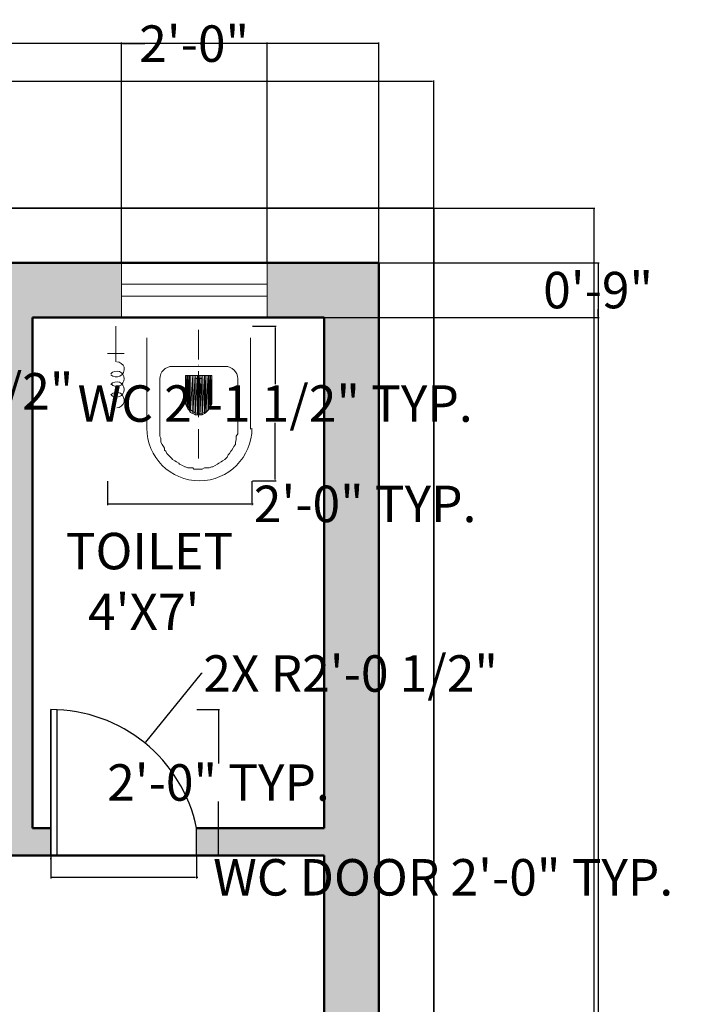
# Model space of a CAD drawing. Units: inches. Extents: x 3398 to 3816, y 15195 to 15771.
# Tile 10 of 10: x 3703 to 3816, y 15609 to 15771. Entities that reach past the tile are written whole.
import ezdxf

# ---------------------------------------------------------------- set-up
doc = ezdxf.new("R2010")
doc.units = ezdxf.units.IN
doc.header["$MEASUREMENT"] = 0
for name, color, linetype, lineweight in [('A-ANNO-DIMS', 2, 'Continuous', 18), ('A-AREA-IDEN', 7, 'Continuous', 25), ('A-DOOR', 3, 'Continuous', 25), ('A-FLOR-FIXT', 8, 'Continuous', 18), ('A-GLAZ', 4, 'Continuous', 18), ('A-WALL', 7, 'Continuous', 50), ('A-WALL-PATT', 252, 'Continuous', 13), ('C-PROP', 7, 'Continuous', 35)]:
    doc.layers.add(name, color=color, linetype=linetype, lineweight=lineweight)
doc.styles.get("Standard").update_dxf_attribs({"font": 'arial.ttf'})
doc.dimstyles.get("Standard").update_dxf_attribs({"dimtxt": 6, "dimasz": 0.18, "dimexe": 0.18, "dimexo": 0.0625, "dimgap": 0.09, "dimtad": 0, "dimtih": 1, "dimtoh": 1, "dimdec": 1, "dimzin": 0, "dimdsep": 46, "dimlunit": 3, "dimtxsty": 'Standard', "dimcen": 0.09, "dimadec": 0, "dimazin": 0, "dimtfac": 1, "dimtdec": 1, "dimtofl": 0, "dimtmove": 0, "dimatfit": 3, "dimfxl": 1, "dimtolj": 1, "dimtzin": 0, "dimarcsym": 0})

# ---------------------------------------------------------------- blocks, each defined once
blk = doc.blocks.new('*D4')
at = {"layer": 'A-ANNO-DIMS', "color": 0, "lineweight": -2, "transparency": 16777216}
for p, q in [((3443.19, 15739.58), (3443.19, 15760.52)), ((3771.19, 15739.58), (3771.19, 15760.52)), ((3443.37, 15760.34), (3593.25, 15760.34)), ((3771.01, 15760.34), (3621.13, 15760.34))]:
    blk.add_line(p, q, dxfattribs=at)
at = {"layer": 'A-ANNO-DIMS', "color": 0, "transparency": 16777216}
for points in [[(3443.37, 15760.37), (3443.37, 15760.31), (3443.19, 15760.34)], [(3771.01, 15760.37), (3771.01, 15760.31), (3771.19, 15760.34)]]:
    blk.add_solid(points, dxfattribs=at)
at = {"layer": 'Defpoints', "color": 0, "transparency": 16777216}
for p in [(3771.19, 15760.34), (3443.19, 15739.52), (3771.19, 15739.52)]:
    blk.add_point(p, dxfattribs=at)
at = {"layer": 'A-ANNO-DIMS', "color": 0, "transparency": 16777216, "insert": (3607.19, 15760.34), "char_height": 6, "attachment_point": 5}
blk.add_mtext('\\A1;27\'-4.0"', dxfattribs=at)
blk = doc.blocks.new('*D5')
at = {"layer": 'A-ANNO-DIMS', "color": 0, "lineweight": -2, "transparency": 16777216}
for p, q in [((3771.25, 15739.52), (3797.69, 15739.52)), ((3797.51, 15739.34), (3797.51, 15488.17)), ((3797.51, 15230.7), (3797.51, 15481.87)), ((3771.25, 15230.52), (3797.69, 15230.52))]:
    blk.add_line(p, q, dxfattribs=at)
at = {"layer": 'A-ANNO-DIMS', "color": 0, "transparency": 16777216}
for points in [[(3797.48, 15739.34), (3797.54, 15739.34), (3797.51, 15739.52)], [(3797.48, 15230.7), (3797.54, 15230.7), (3797.51, 15230.52)]]:
    blk.add_solid(points, dxfattribs=at)
at = {"layer": 'Defpoints', "color": 0, "transparency": 16777216}
for p in [(3771.19, 15739.52), (3771.19, 15230.52), (3797.51, 15230.52)]:
    blk.add_point(p, dxfattribs=at)
at = {"layer": 'A-ANNO-DIMS', "color": 0, "transparency": 16777216, "insert": (3797.51, 15485.02), "char_height": 6, "attachment_point": 5}
blk.add_mtext('\\A1;42\'-5.0"', dxfattribs=at)
blk = doc.blocks.new('WC-PLAN')
h = blk.add_hatch(color=256)
h.paths.add_polyline_path([(12.84, 17.3), (12.84, 12.59), (13.07, 17.3)])
h.paths.add_polyline_path([(12.84, 12.59), (13.07, 17.3), (13.07, 12.21)])
h = blk.add_hatch(color=256)
h.paths.add_polyline_path([(13.07, 17.3), (13.07, 12.21), (13.22, 17.3)])
h.paths.add_polyline_path([(13.07, 12.21), (13.22, 17.3), (13.22, 11.83)])
h = blk.add_hatch(color=256)
h.paths.add_polyline_path([(13.22, 17.3), (13.22, 11.83), (13.45, 17.3)])
h.paths.add_polyline_path([(13.22, 11.83), (13.45, 17.3), (13.45, 11.61)])
h = blk.add_hatch(color=256)
h.paths.add_polyline_path([(13.45, 17.3), (13.45, 11.61), (13.6, 17.3)])
h.paths.add_polyline_path([(13.45, 11.61), (13.6, 17.3), (13.6, 11.23)])
h = blk.add_hatch(color=256)
h.paths.add_polyline_path([(13.6, 17.3), (13.6, 11.23), (14.06, 17.3)])
h.paths.add_polyline_path([(13.6, 11.23), (14.06, 17.3), (14.06, 11.08)])
h = blk.add_hatch(color=256)
h.paths.add_polyline_path([(14.06, 17.3), (14.06, 11.08), (14.44, 17.3)])
h.paths.add_polyline_path([(14.06, 11.08), (14.44, 17.3), (14.44, 10.85)])
h = blk.add_hatch(color=256)
h.paths.add_polyline_path([(14.44, 17.3), (14.44, 10.85), (14.82, 17.3)])
h.paths.add_polyline_path([(14.44, 10.85), (14.82, 17.3), (14.82, 10.85)])
h = blk.add_hatch(color=256)
h.paths.add_polyline_path([(14.82, 17.3), (14.82, 10.85), (15.19, 17.3)])
h.paths.add_polyline_path([(14.82, 10.85), (15.19, 17.3), (15.2, 10.85)])
h = blk.add_hatch(color=256)
h.paths.add_polyline_path([(15.19, 17.3), (15.2, 10.85), (15.57, 17.3)])
h.paths.add_polyline_path([(15.2, 10.85), (15.57, 17.3), (15.58, 10.85)])
h = blk.add_hatch(color=256)
h.paths.add_polyline_path([(15.57, 17.3), (15.58, 10.85), (15.95, 17.3)])
h.paths.add_polyline_path([(15.58, 10.85), (15.95, 17.3), (15.96, 11.08)])
h = blk.add_hatch(color=256)
h.paths.add_polyline_path([(15.95, 17.3), (15.96, 11.08), (16.18, 17.3)])
h.paths.add_polyline_path([(15.96, 11.08), (16.18, 17.3), (16.18, 11.23)])
h = blk.add_hatch(color=256)
h.paths.add_polyline_path([(16.18, 17.3), (16.18, 11.23), (16.56, 17.3)])
h.paths.add_polyline_path([(16.18, 11.23), (16.56, 17.3), (16.56, 11.61)])
h = blk.add_hatch(color=256)
h.paths.add_polyline_path([(16.56, 17.3), (16.56, 11.61), (16.71, 17.3)])
h.paths.add_polyline_path([(16.56, 11.61), (16.71, 17.3), (16.71, 11.83)])
h = blk.add_hatch(color=256)
h.paths.add_polyline_path([(16.71, 17.3), (16.71, 11.83), (16.94, 17.3)])
h.paths.add_polyline_path([(16.71, 11.83), (16.94, 17.3), (16.94, 12.21)])
h = blk.add_hatch(color=256)
h.paths.add_polyline_path([(16.94, 17.3), (16.94, 12.21), (17.17, 17.3)])
h.paths.add_polyline_path([(16.94, 12.21), (17.17, 17.3), (17.17, 12.59)])
h.paths.add_polyline_path([(17.17, 17.3), (17.17, 12.59), (17.17, 12.97)])
for points in [[(1.36, 25.41), (1.37, 19.57), (1.37, 19.57)], [(14.97, 24.81), (14.97, 19.95), (14.97, 19.95)], [(6.47, 23.51), (6.47, 8.49), (6.47, 8.49)], [(23.54, 23.52), (23.54, 8.5), (23.54, 8.5)], [(2.73, 20.93), (0, 20.93), (0, 20.93)], [(19.29, 18.81), (10.57, 18.81), (10.57, 18.81)], [(14.97, 19.04), (15.04, 19.04), (15.04, 19.04)], [(14.97, 18.05), (14.97, 10.47), (14.97, 10.47)], [(8.6, 16.69), (8.6, 9.48), (8.6, 9.48)], [(17.17, 17.3), (12.84, 17.3), (12.84, 17.3)], [(12.84, 17.3), (12.84, 12.97), (12.84, 12.97)], [(14.59, 16.84), (14.59, 16.92), (14.59, 16.92)], [(14.97, 16.84), (14.82, 16.84), (14.59, 16.84)], [(14.97, 16.84), (15.04, 16.92), (15.04, 16.92)], [(15.42, 16.84), (15.2, 16.84), (14.97, 16.84)], [(15.42, 16.84), (15.42, 16.92), (15.42, 16.92)], [(17.17, 17.3), (17.17, 12.97), (17.17, 12.97)], [(21.42, 16.69), (21.42, 9.48), (21.42, 9.48)], [(21.42, 9.48), (21.42, 8.73), (21.42, 8.12), (21.42, 7.74), (21.19, 7.36), (21.19, 6.98), (21.19, 6.75), (21.04, 6.37), (21.04, 5.99), (20.81, 5.62), (20.66, 5.39), (20.43, 5.01), (20.28, 4.86), (20.05, 4.48), (19.83, 4.25), (19.67, 3.87), (19.45, 3.64), (19.29, 3.49), (18.92, 3.26), (18.69, 3.11), (18.31, 2.88), (18.08, 2.73), (17.7, 2.5), (17.32, 2.28), (17.17, 2.28), (16.72, 2.12), (16.34, 2.12), (15.96, 2.12), (15.58, 1.9), (14.97, 1.9), (14.21, 1.9), (14.06, 2.12), (13.61, 2.12), (13.23, 2.12), (12.85, 2.28), (12.7, 2.28), (12.32, 2.5), (11.86, 2.73), (11.71, 2.88), (11.33, 3.11), (11.1, 3.26), (10.72, 3.49), (10.57, 3.64), (10.34, 3.87), (9.96, 4.25), (9.74, 4.47), (9.58, 4.85), (9.36, 5.01), (9.36, 5.38), (9.21, 5.61), (8.98, 5.99), (8.75, 6.37), (8.75, 6.75), (8.75, 6.98), (8.6, 7.36), (8.6, 7.74), (8.6, 8.12), (8.6, 8.72), (8.6, 9.48)], [(14.97, 8.5), (14.97, 3.64), (14.97, 3.64)]]:
    blk.add_lwpolyline(points)
for points in [[(12.84, 17.3), (12.84, 12.97)], [(12.84, 12.97), (12.84, 17.3), (12.84, 12.59)], [(12.84, 17.3), (12.84, 12.59), (13.07, 17.3)], [(12.84, 12.59), (13.07, 17.3), (13.07, 12.21)], [(13.07, 17.3), (13.07, 12.21), (13.22, 17.3)], [(13.07, 12.21), (13.22, 17.3), (13.22, 11.83)], [(13.22, 17.3), (13.22, 11.83), (13.45, 17.3)], [(13.22, 11.83), (13.45, 17.3), (13.45, 11.61)], [(13.45, 17.3), (13.45, 11.61), (13.6, 17.3)], [(13.45, 11.61), (13.6, 17.3), (13.6, 11.23)], [(13.6, 17.3), (13.6, 11.23), (14.06, 17.3)], [(13.6, 11.23), (14.06, 17.3), (14.06, 11.08)], [(14.06, 17.3), (14.06, 11.08), (14.44, 17.3)], [(14.06, 11.08), (14.44, 17.3), (14.44, 10.85)], [(14.44, 17.3), (14.44, 10.85), (14.82, 17.3)], [(14.44, 10.85), (14.82, 17.3), (14.82, 10.85)], [(14.82, 17.3), (14.82, 10.85), (15.19, 17.3)], [(14.82, 10.85), (15.19, 17.3), (15.2, 10.85)], [(15.19, 17.3), (15.2, 10.85), (15.57, 17.3)], [(15.2, 10.85), (15.57, 17.3), (15.58, 10.85)], [(15.57, 17.3), (15.58, 10.85), (15.95, 17.3)], [(15.58, 10.85), (15.95, 17.3), (15.96, 11.08)], [(15.95, 17.3), (15.96, 11.08), (16.18, 17.3)], [(15.96, 11.08), (16.18, 17.3), (16.18, 11.23)], [(16.18, 17.3), (16.18, 11.23), (16.56, 17.3)], [(16.18, 11.23), (16.56, 17.3), (16.56, 11.61)], [(16.56, 17.3), (16.56, 11.61), (16.71, 17.3)], [(16.56, 11.61), (16.71, 17.3), (16.71, 11.83)], [(16.71, 17.3), (16.71, 11.83), (16.94, 17.3)], [(16.71, 11.83), (16.94, 17.3), (16.94, 12.21)], [(16.94, 17.3), (16.94, 12.21), (17.17, 17.3)], [(16.94, 12.21), (17.17, 17.3), (17.17, 12.59)], [(17.17, 17.3), (17.17, 12.59), (17.17, 12.97)], [(17.17, 12.59), (17.17, 17.3), (17.17, 17.3)]]:
    blk.add_lwpolyline(points, close=True)
for points, knots in [([(0.53, 17.44), (0.91, 17.06), (1.59, 16.91), (2.05, 17.22), (2.05, 17.22), (2.58, 17.52), (2.88, 18.05), (2.73, 18.66), (2.73, 18.66), (2.58, 19.19), (2.05, 19.57), (1.52, 19.57)], [0, 0, 0, 0, 0.083333, 0.083333, 0.083333, 0.083334, 0.166667, 0.166667, 0.166667, 0.166668, 1, 1, 1, 1]), ([(0.61, 15.93), (0.91, 15.55), (1.52, 15.4), (1.97, 15.62), (1.97, 15.62), (2.43, 15.78), (2.73, 16.31), (2.73, 16.76), (2.73, 16.76), (2.73, 17.29), (2.43, 17.75), (1.97, 17.97), (1.97, 17.97), (1.44, 18.13), (0.91, 17.97), (0.53, 17.6)], [0, 0, 0, 0, 0.0625, 0.0625, 0.0625, 0.062501, 0.125, 0.125, 0.125, 0.125001, 0.1875, 0.1875, 0.1875, 0.187501, 1, 1, 1, 1]), ([(0.53, 14.18), (0.91, 13.8), (1.44, 13.65), (1.97, 13.88), (1.97, 13.88), (2.43, 14.03), (2.73, 14.49), (2.73, 15.02), (2.73, 15.02), (2.73, 15.55), (2.43, 16), (1.97, 16.23), (1.97, 16.23), (1.44, 16.38), (0.91, 16.23), (0.53, 15.85)], [0, 0, 0, 0, 0.0625, 0.0625, 0.0625, 0.062501, 0.125, 0.125, 0.125, 0.125001, 0.1875, 0.1875, 0.1875, 0.187501, 1, 1, 1, 1]), ([(1.52, 11.98), (2.05, 11.98), (2.58, 12.44), (2.73, 12.97), (2.73, 12.97), (2.88, 13.5), (2.58, 14.11), (2.13, 14.41), (2.13, 14.41), (1.59, 14.64), (0.99, 14.56), (0.61, 14.18)], [0, 0, 0, 0, 0.083333, 0.083333, 0.083333, 0.083334, 0.166667, 0.166667, 0.166667, 0.166668, 1, 1, 1, 1]), ([(13.07, 13.12), (13.07, 11.99), (13.98, 11.08), (15.12, 11.08), (15.12, 11.08), (16.26, 11.08), (17.17, 11.99), (17.17, 13.12)], [0, 0, 0, 0, 0.125, 0.125, 0.125, 0.125001, 1, 1, 1, 1]), ([(6.47, 8.65), (6.47, 3.87), (10.34, 0), (15.12, 0), (15.12, 0), (19.9, 0), (23.77, 3.87), (23.77, 8.65)], [0, 0, 0, 0, 0.125, 0.125, 0.125, 0.125001, 1, 1, 1, 1])]:
    blk.add_open_spline(points, degree=3, knots=knots)
for points in [[(10.64, 18.81), (9.51, 18.81), (8.6, 17.9), (8.6, 16.76)], [(21.42, 16.77), (21.42, 17.9), (20.5, 18.81), (19.37, 18.81)]]:
    blk.add_open_spline(points, degree=3)
blk = doc.blocks.new('DOOR-SWING-24IN')
for p, q in [((0, 0), (0, 24)), ((1, 24), (1, 0)), ((0, 0), (24, 0))]:
    blk.add_line(p, q)
blk.add_arc((0, -0.52), 24.52, 11.8123, 90)
blk = doc.blocks.new('*D24')
at = {"layer": 'A-ANNO-DIMS', "color": 0, "lineweight": -2, "transparency": 16777216}
for p, q in [((3741.36, 15720.07), (3745.29, 15720.07)), ((3745.11, 15719.89), (3745.11, 15710.56)), ((3745.11, 15694.84), (3745.11, 15704.17)), ((3741.36, 15694.66), (3745.29, 15694.66))]:
    blk.add_line(p, q, dxfattribs=at)
at = {"layer": 'A-ANNO-DIMS', "color": 0, "transparency": 16777216}
for points in [[(3745.08, 15719.89), (3745.14, 15719.89), (3745.11, 15720.07)], [(3745.08, 15694.84), (3745.14, 15694.84), (3745.11, 15694.66)]]:
    blk.add_solid(points, dxfattribs=at)
at = {"layer": 'Defpoints', "color": 0, "transparency": 16777216}
for p in [(3741.3, 15720.07), (3745.11, 15720.07), (3741.3, 15694.66)]:
    blk.add_point(p, dxfattribs=at)
at = {"layer": 'A-ANNO-DIMS', "color": 0, "transparency": 16777216, "insert": (3745.11, 15707.36), "char_height": 6, "attachment_point": 5}
blk.add_mtext('\\A1;WC 2\'-1 1/2" TYP.', dxfattribs=at)
blk = doc.blocks.new('*D25')
at = {"layer": 'A-ANNO-DIMS', "color": 0, "lineweight": -2, "transparency": 16777216}
for p, q in [((3717.53, 15694.6), (3717.53, 15690.67)), ((3741.3, 15694.6), (3741.3, 15690.67)), ((3717.71, 15690.85), (3741.12, 15690.85)), ((3741.3, 15690.85), (3741.48, 15690.85))]:
    blk.add_line(p, q, dxfattribs=at)
at = {"layer": 'A-ANNO-DIMS', "color": 0, "transparency": 16777216}
for points in [[(3717.71, 15690.88), (3717.71, 15690.82), (3717.53, 15690.85)], [(3741.12, 15690.88), (3741.12, 15690.82), (3741.3, 15690.85)]]:
    blk.add_solid(points, dxfattribs=at)
at = {"layer": 'Defpoints', "color": 0, "transparency": 16777216}
for p in [(3717.53, 15694.66), (3741.3, 15694.66), (3741.3, 15690.85)]:
    blk.add_point(p, dxfattribs=at)
at = {"layer": 'A-ANNO-DIMS', "color": 0, "transparency": 16777216, "insert": (3759.91, 15690.85), "char_height": 6, "attachment_point": 5}
blk.add_mtext('\\A1;2\'-0" TYP.', dxfattribs=at)
blk = doc.blocks.new('*D28')
at = {"layer": 'A-ANNO-DIMS', "color": 0, "lineweight": -2, "transparency": 16777216}
for p, q in [((3708.19, 15632.96), (3708.19, 15629.24)), ((3732.19, 15632.96), (3732.19, 15629.24)), ((3708.37, 15629.42), (3732.01, 15629.42)), ((3732.19, 15629.42), (3732.37, 15629.42))]:
    blk.add_line(p, q, dxfattribs=at)
at = {"layer": 'A-ANNO-DIMS', "color": 0, "transparency": 16777216}
for points in [[(3708.37, 15629.45), (3708.37, 15629.39), (3708.19, 15629.42)], [(3732.01, 15629.45), (3732.01, 15629.39), (3732.19, 15629.42)]]:
    blk.add_solid(points, dxfattribs=at)
at = {"layer": 'Defpoints', "color": 0, "transparency": 16777216}
for p in [(3708.19, 15633.02), (3732.19, 15633.02), (3732.19, 15629.42)]:
    blk.add_point(p, dxfattribs=at)
at = {"layer": 'A-ANNO-DIMS', "color": 0, "transparency": 16777216, "insert": (3772.75, 15629.42), "char_height": 6, "attachment_point": 5}
blk.add_mtext('\\A1;WC DOOR 2\'-0" TYP.', dxfattribs=at)
blk = doc.blocks.new('*D29')
at = {"layer": 'A-ANNO-DIMS', "color": 0, "lineweight": -2, "transparency": 16777216}
for p, q in [((3732.25, 15657.02), (3735.97, 15657.02)), ((3735.79, 15656.84), (3735.79, 15648.17)), ((3735.79, 15633.2), (3735.79, 15641.87)), ((3732.25, 15633.02), (3735.97, 15633.02))]:
    blk.add_line(p, q, dxfattribs=at)
at = {"layer": 'A-ANNO-DIMS', "color": 0, "transparency": 16777216}
for points in [[(3735.76, 15656.84), (3735.82, 15656.84), (3735.79, 15657.02)], [(3735.76, 15633.2), (3735.82, 15633.2), (3735.79, 15633.02)]]:
    blk.add_solid(points, dxfattribs=at)
at = {"layer": 'Defpoints', "color": 0, "transparency": 16777216}
for p in [(3732.19, 15657.02), (3735.79, 15657.02), (3732.19, 15633.02)]:
    blk.add_point(p, dxfattribs=at)
at = {"layer": 'A-ANNO-DIMS', "color": 0, "transparency": 16777216, "insert": (3735.79, 15645.02), "char_height": 6, "attachment_point": 5}
blk.add_mtext('\\A1;2\'-0" TYP.', dxfattribs=at)
blk = doc.blocks.new('*D36')
at = {"layer": 'A-ANNO-DIMS', "color": 0, "lineweight": -2, "transparency": 16777216}
for p, q in [((3465.19, 15730.58), (3465.19, 15766.75)), ((3465.37, 15766.57), (3603.24, 15766.57)), ((3762.01, 15766.57), (3624.14, 15766.57)), ((3762.19, 15730.58), (3762.19, 15766.75))]:
    blk.add_line(p, q, dxfattribs=at)
at = {"layer": 'A-ANNO-DIMS', "color": 0, "transparency": 16777216}
for points in [[(3465.37, 15766.6), (3465.37, 15766.54), (3465.19, 15766.57)], [(3762.01, 15766.6), (3762.01, 15766.54), (3762.19, 15766.57)]]:
    blk.add_solid(points, dxfattribs=at)
at = {"layer": 'Defpoints', "color": 0, "transparency": 16777216}
for p in [(3762.19, 15766.57), (3465.19, 15730.52), (3762.19, 15730.52)]:
    blk.add_point(p, dxfattribs=at)
at = {"layer": 'A-ANNO-DIMS', "color": 0, "transparency": 16777216, "insert": (3613.69, 15766.57), "char_height": 6, "attachment_point": 5}
blk.add_mtext('\\A1;24\'-9"', dxfattribs=at)
blk = doc.blocks.new('*D37')
at = {"layer": 'A-ANNO-DIMS', "color": 0, "lineweight": -2, "transparency": 16777216}
for p, q in [((3762.25, 15730.52), (3798.42, 15730.52)), ((3798.24, 15730.34), (3798.24, 15525.96)), ((3798.24, 15315.2), (3798.24, 15519.58)), ((3762.25, 15315.02), (3798.42, 15315.02))]:
    blk.add_line(p, q, dxfattribs=at)
at = {"layer": 'A-ANNO-DIMS', "color": 0, "transparency": 16777216}
for points in [[(3798.21, 15730.34), (3798.27, 15730.34), (3798.24, 15730.52)], [(3798.21, 15315.2), (3798.27, 15315.2), (3798.24, 15315.02)]]:
    blk.add_solid(points, dxfattribs=at)
at = {"layer": 'Defpoints', "color": 0, "transparency": 16777216}
for p in [(3762.19, 15730.52), (3798.24, 15730.52), (3762.19, 15315.02)]:
    blk.add_point(p, dxfattribs=at)
at = {"layer": 'A-ANNO-DIMS', "color": 0, "transparency": 16777216, "insert": (3798.24, 15522.77), "char_height": 6, "attachment_point": 5}
blk.add_mtext('\\A1;34\'-7 1/2"', dxfattribs=at)
blk = doc.blocks.new('*D43')
at = {"layer": 'A-ANNO-DIMS', "color": 0, "lineweight": -2, "transparency": 16777216}
for p, q in [((3762.25, 15730.52), (3798.42, 15730.52)), ((3798.24, 15730.34), (3798.24, 15729.17)), ((3798.24, 15721.7), (3798.24, 15722.87)), ((3753.25, 15721.52), (3798.42, 15721.52))]:
    blk.add_line(p, q, dxfattribs=at)
at = {"layer": 'A-ANNO-DIMS', "color": 0, "transparency": 16777216}
for points in [[(3798.21, 15730.34), (3798.27, 15730.34), (3798.24, 15730.52)], [(3798.21, 15721.7), (3798.27, 15721.7), (3798.24, 15721.52)]]:
    blk.add_solid(points, dxfattribs=at)
at = {"layer": 'Defpoints', "color": 0, "transparency": 16777216}
for p in [(3762.19, 15730.52), (3753.19, 15721.52), (3798.24, 15721.52)]:
    blk.add_point(p, dxfattribs=at)
at = {"layer": 'A-ANNO-DIMS', "color": 0, "transparency": 16777216, "insert": (3798.24, 15726.02), "char_height": 6, "attachment_point": 5}
blk.add_mtext('\\A1;0\'-9"', dxfattribs=at)
blk = doc.blocks.new('*D48')
at = {"layer": 'A-ANNO-DIMS', "color": 0, "lineweight": -2, "transparency": 16777216}
for p, q in [((3719.81, 15730.58), (3719.81, 15766.75)), ((3719.99, 15766.57), (3723.67, 15766.57)), ((3743.59, 15766.57), (3739.9, 15766.57)), ((3743.77, 15730.58), (3743.77, 15766.75))]:
    blk.add_line(p, q, dxfattribs=at)
at = {"layer": 'A-ANNO-DIMS', "color": 0, "transparency": 16777216}
for points in [[(3719.99, 15766.6), (3719.99, 15766.54), (3719.81, 15766.57)], [(3743.59, 15766.6), (3743.59, 15766.54), (3743.77, 15766.57)]]:
    blk.add_solid(points, dxfattribs=at)
at = {"layer": 'Defpoints', "color": 0, "transparency": 16777216}
for p in [(3743.77, 15766.57), (3719.81, 15730.52), (3743.77, 15730.52)]:
    blk.add_point(p, dxfattribs=at)
at = {"layer": 'A-ANNO-DIMS', "color": 0, "transparency": 16777216, "insert": (3731.79, 15766.57), "char_height": 6, "attachment_point": 5}
blk.add_mtext('\\A1;2\'-0"', dxfattribs=at)
blk = doc.blocks.new('*D57')
at = {"layer": 'A-ANNO-DIMS', "color": 0, "lineweight": -2, "transparency": 16777216}
for p, q in [((3732.93, 15662.95), (3723.76, 15651.67)), ((3733.11, 15662.95), (3732.93, 15662.95)), ((3708.19, 15632.41), (3708.19, 15632.59)), ((3708.1, 15632.5), (3708.28, 15632.5))]:
    blk.add_line(p, q, dxfattribs=at)
at = {"layer": 'A-ANNO-DIMS', "color": 0, "transparency": 16777216}
blk.add_solid([(3723.74, 15651.69), (3723.79, 15651.65), (3723.65, 15651.53)], dxfattribs=at)
at = {"layer": 'Defpoints', "color": 0, "transparency": 16777216}
for p in [(3723.65, 15651.53), (3708.19, 15632.5)]:
    blk.add_point(p, dxfattribs=at)
at = {"layer": 'A-ANNO-DIMS', "color": 0, "transparency": 16777216, "insert": (3757.53, 15662.95), "char_height": 6, "attachment_point": 5}
blk.add_mtext('\\A1;2X R2\'-0 1/2"', dxfattribs=at)
blk = doc.blocks.new('*D59')
at = {"layer": 'A-ANNO-DIMS', "color": 0, "lineweight": -2, "transparency": 16777216}
for p, q in [((3614.32, 15709.48), (3614.5, 15709.48)), ((3614.41, 15709.39), (3614.41, 15709.57)), ((3663.27, 15709.37), (3645.13, 15709.41))]:
    blk.add_line(p, q, dxfattribs=at)
at = {"layer": 'A-ANNO-DIMS', "color": 0, "transparency": 16777216}
blk.add_solid([(3645.13, 15709.44), (3645.13, 15709.38), (3644.95, 15709.41)], dxfattribs=at)
at = {"layer": 'Defpoints', "color": 0, "transparency": 16777216}
for p in [(3614.41, 15709.48), (3644.95, 15709.41)]:
    blk.add_point(p, dxfattribs=at)
at = {"layer": 'A-ANNO-DIMS', "color": 0, "transparency": 16777216, "insert": (3687.69, 15709.37), "char_height": 6, "attachment_point": 5}
blk.add_mtext('\\A1;2X R2\'-6 1/2"', dxfattribs=at)

msp = doc.modelspace()

# ---------------------------------------------------------------- hatches: boundary and pattern name
at = {"layer": 'A-WALL-PATT'}
h = msp.add_hatch(color=256, dxfattribs=at)
h.dxf.hatch_style = 1
h.paths.add_polyline_path([(3515.96, 15730.52), (3465.19, 15730.52), (3465.19, 15715.52), (3474.19, 15715.52), (3474.19, 15721.52), (3515.96, 15721.52)])
h.paths.add_polyline_path([(3719.81, 15730.52), (3675.76, 15730.52), (3675.76, 15721.52), (3700.69, 15721.52), (3700.69, 15637.52), (3610.69, 15637.52), (3610.69, 15663.97), (3606.19, 15663.97), (3606.19, 15601.52), (3599.08, 15601.52), (3599.08, 15592.52), (3606.19, 15592.52), (3606.19, 15508.52), (3616.69, 15508.52), (3616.69, 15513.02), (3610.69, 15513.02), (3610.69, 15633.02), (3708.19, 15633.02), (3708.19, 15637.52), (3705.19, 15637.52), (3705.19, 15721.52), (3719.81, 15721.52)])
h.paths.add_polyline_path([(3762.19, 15730.52), (3743.77, 15730.52), (3743.77, 15721.52), (3753.19, 15721.52), (3753.19, 15637.52), (3732.19, 15637.52), (3732.19, 15633.02), (3753.19, 15633.02), (3753.19, 15597.39), (3762.19, 15597.39)])
h.paths.add_polyline_path([(3762.19, 15549.39), (3753.19, 15549.39), (3753.19, 15513.02), (3652.69, 15513.02), (3652.69, 15508.52), (3664.69, 15508.52), (3664.69, 15460.52), (3652.69, 15460.52), (3652.69, 15456.02), (3672.19, 15456.02), (3672.19, 15460.52), (3669.19, 15460.52), (3669.19, 15508.52), (3753.19, 15508.52), (3753.19, 15497.51), (3762.19, 15497.51)])
h.paths.add_polyline_path([(3762.19, 15473.48), (3753.19, 15473.48), (3753.19, 15460.52), (3696.19, 15460.52), (3696.19, 15456.02), (3753.19, 15456.02), (3753.19, 15414.25), (3762.19, 15414.25)])
h.paths.add_polyline_path([(3762.19, 15366.28), (3753.19, 15366.28), (3753.19, 15324.02), (3610.69, 15324.02), (3610.69, 15456.02), (3616.69, 15456.02), (3616.69, 15460.52), (3610.69, 15460.52), (3606.19, 15460.52), (3606.19, 15382.52), (3587.73, 15382.52), (3587.73, 15373.52), (3606.19, 15373.52), (3606.19, 15315.02), (3762.19, 15315.02)])
h.paths.add_polyline_path([(3539.73, 15382.52), (3522.19, 15382.52), (3522.19, 15373.52), (3539.73, 15373.52)])
h.paths.add_polyline_path([(3480.19, 15382.52), (3474.19, 15382.52), (3474.19, 15452.47), (3465.19, 15452.47), (3465.19, 15373.52), (3480.19, 15373.52)])
h.paths.add_polyline_path([(3551.04, 15601.52), (3474.19, 15601.52), (3474.19, 15679.52), (3465.19, 15679.52), (3465.19, 15500.47), (3474.19, 15500.47), (3474.19, 15592.52), (3551.04, 15592.52)])

# ---------------------------------------------------------------- linework, layer by layer
at = {"layer": 'A-DOOR'}
for p, q in [((3708.19, 15657.02), (3708.19, 15633.02)), ((3732.19, 15633.02), (3732.19, 15637.52)), ((3705.19, 15633.02), (3708.19, 15633.02))]:
    msp.add_line(p, q, dxfattribs=at)
at = {"layer": 'A-GLAZ'}
for p, q in [((3719.81, 15730.52), (3719.81, 15721.52)), ((3743.77, 15730.52), (3719.81, 15730.52)), ((3743.77, 15721.52), (3743.77, 15730.52)), ((3743.77, 15727.02), (3719.81, 15727.02)), ((3719.81, 15725.02), (3743.77, 15725.02)), ((3719.81, 15721.52), (3743.77, 15721.52))]:
    msp.add_line(p, q, dxfattribs=at)
at = {"layer": 'A-WALL'}
for p, q in [((3452.19, 15730.52), (3762.19, 15730.52)), ((3762.19, 15730.52), (3762.19, 15230.52)), ((3705.19, 15721.52), (3705.19, 15637.52)), ((3705.19, 15721.52), (3753.19, 15721.52)), ((3753.19, 15721.52), (3753.19, 15637.52)), ((3705.19, 15637.52), (3708.19, 15637.52)), ((3732.19, 15637.52), (3753.19, 15637.52)), ((3610.69, 15633.02), (3753.19, 15633.02)), ((3753.19, 15633.02), (3753.19, 15513.02))]:
    msp.add_line(p, q, dxfattribs=at)
at = {"layer": 'C-PROP'}
for p, q in [((3443.19, 15739.52), (3771.19, 15739.52)), ((3771.19, 15739.52), (3771.19, 15230.52))]:
    msp.add_line(p, q, dxfattribs=at)

# ---------------------------------------------------------------- block references
at = {"layer": 'A-DOOR'}
msp.add_blockref('DOOR-SWING-24IN', (3708.19, 15633.02), dxfattribs=at)
at = {"layer": 'A-FLOR-FIXT'}
msp.add_blockref('WC-PLAN', (3717.53, 15694.66), dxfattribs=at)

# ---------------------------------------------------------------- texts
at = {"layer": 'A-AREA-IDEN', "insert": (3710.66, 15686.09), "char_height": 6, "attachment_point": 1}
msp.add_mtext_dynamic_manual_height_columns("TOILET\\P  4'X7'", width=32.3129, gutter_width=30, heights=[0], dxfattribs=at)

# ---------------------------------------------------------------- dimensions: what is measured, and where the dimension line sits
at = {"layer": 'A-ANNO-DIMS'}
for base, p1, p2, override, picture, middle in [((3762.19, 15766.57), (3465.19, 15730.52), (3762.19, 15730.52), {"dimdec": 1, "dimlfac": 1, "dimrnd": 0, "dimzin": 1, "dimdsep": 46, "dimlunit": 4, "dimfrac": 2}, '*D36', (3613.69, 15766.57)), ((3743.77, 15766.57), (3719.81, 15730.52), (3743.77, 15730.52), {"dimdec": 1, "dimlfac": 1, "dimrnd": 0, "dimzin": 1, "dimdsep": 46, "dimlunit": 4, "dimfrac": 2}, '*D48', (3731.79, 15766.57)), ((3771.19, 15760.34), (3443.19, 15739.52), (3771.19, 15739.52), {"dimclrd": 0, "dimclre": 0, "dimclrt": 0}, '*D4', (3607.19, 15760.34))]:
    dim = msp.add_linear_dim(base=base, p1=p1, p2=p2, dimstyle='Standard', override=override, dxfattribs=at)
    dim.commit()
    dim.dimension.update_dxf_attribs({"geometry": picture, "text_midpoint": middle})
for base, p1, p2, override, picture, middle in [((3797.51, 15230.52), (3771.19, 15739.52), (3771.19, 15230.52), {"dimclrd": 0, "dimclre": 0, "dimclrt": 0}, '*D5', (3797.51, 15485.02)), ((3798.24, 15721.52), (3762.19, 15730.52), (3753.19, 15721.52), {"dimdec": 1, "dimlfac": 1, "dimrnd": 0, "dimzin": 1, "dimdsep": 46, "dimlunit": 4, "dimfrac": 2}, '*D43', (3798.24, 15726.02)), ((3798.24, 15730.52), (3762.19, 15315.02), (3762.19, 15730.52), {"dimdec": 1, "dimlfac": 1, "dimrnd": 0, "dimzin": 1, "dimdsep": 46, "dimlunit": 4, "dimfrac": 2}, '*D37', (3798.24, 15522.77))]:
    dim = msp.add_linear_dim(base=base, p1=p1, p2=p2, angle=90, dimstyle='Standard', override=override, dxfattribs=at)
    dim.commit()
    dim.dimension.update_dxf_attribs({"geometry": picture, "text_midpoint": middle})
for base, p1, p2, text, picture, middle in [((3745.11, 15720.07), (3741.3, 15694.66), (3741.3, 15720.07), 'WC <> TYP.', '*D24', (3745.11, 15707.36)), ((3735.79, 15657.02), (3732.19, 15633.02), (3732.19, 15657.02), '<> TYP.', '*D29', (3735.79, 15645.02))]:
    dim = msp.add_linear_dim(base=base, p1=p1, p2=p2, angle=90, text=text, dimstyle='Standard', override={"dimdec": 1, "dimlfac": 1, "dimrnd": 0, "dimzin": 1, "dimdsep": 46, "dimlunit": 4, "dimfrac": 2}, dxfattribs=at)
    dim.commit()
    dim.dimension.update_dxf_attribs({"geometry": picture, "text_midpoint": middle})
for center, mpoint, picture, middle in [((3614.41, 15709.48), (3644.95, 15709.41), '*D59', (3663.27, 15709.37)), ((3708.19, 15632.5), (3723.65, 15651.53), '*D57', (3757.53, 15662.95))]:
    dim = msp.add_radius_dim(center=center, mpoint=mpoint, text='2X <>', dimstyle='Standard', override={"dimdec": 1, "dimlfac": 1, "dimrnd": 0, "dimzin": 1, "dimdsep": 46, "dimlunit": 4, "dimfrac": 2}, dxfattribs=at)
    dim.commit()
    dim.dimension.update_dxf_attribs({"geometry": picture, "text_midpoint": middle, "dimtype": 164})
for base, p1, p2, text, picture, middle in [((3741.3, 15690.85), (3717.53, 15694.66), (3741.3, 15694.66), '<> TYP.', '*D25', (3759.91, 15690.85)), ((3732.19, 15629.42), (3708.19, 15633.02), (3732.19, 15633.02), 'WC DOOR <> TYP.', '*D28', (3772.75, 15629.42))]:
    dim = msp.add_linear_dim(base=base, p1=p1, p2=p2, text=text, dimstyle='Standard', override={"dimdec": 1, "dimlfac": 1, "dimrnd": 0, "dimzin": 1, "dimdsep": 46, "dimlunit": 4, "dimfrac": 2}, dxfattribs=at)
    dim.commit()
    dim.dimension.update_dxf_attribs({"geometry": picture, "text_midpoint": middle})

doc.saveas('drawing.dxf')
